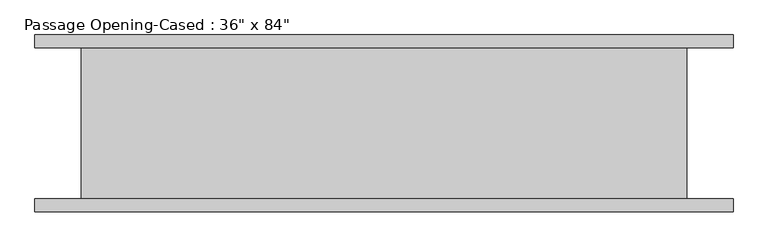
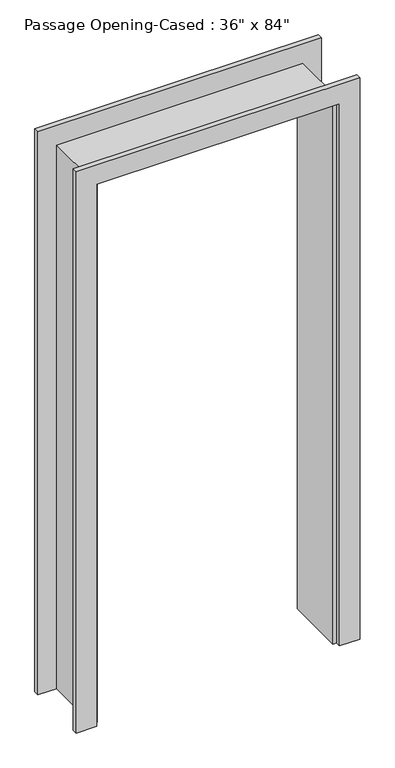
"""IFC4 building model written with IfcOpenShell, lengths in millimetres: proxy geometry."""

from ifc_helpers import new_model, si_unit, frame, origin, place, context, project, spatial, polyline, outline, extrude, faceted_brep, source, transform, mapped, element, save


def proxy_e9bf662a(model_context):
    return source(origin(), model_context, "Body", "SolidModel", [
        faceted_brep([(429.9613433, 114.3, 0.0), (449.0113433, 114.3, 0.0), (449.0113433, -114.3, 0.0), (429.9613433, -114.3, 0.0), (429.9613433, 114.3, 2114.55), (449.0113433, 114.3, 2133.6), (449.0113433, -114.3, 2133.6), (429.9613433, -114.3, 2114.55), (-446.3386567, 114.3, 2114.55), (-465.3886567, 114.3, 2133.6), (-465.3886567, -114.3, 2133.6), (-446.3386567, -114.3, 2114.55), (-446.3386567, 114.3, 0.0), (-446.3386567, -114.3, 0.0), (-465.3886567, -114.3, 0.0), (-465.3886567, 114.3, 0.0)], [[[0, 1, 2, 3]], [[1, 0, 4, 5]], [[2, 1, 5, 6]], [[3, 2, 6, 7]], [[0, 3, 7, 4]], [[5, 4, 8, 9]], [[6, 5, 9, 10]], [[7, 6, 10, 11]], [[4, 7, 11, 8]], [[12, 13, 14, 15]], [[9, 8, 12, 15]], [[10, 9, 15, 14]], [[11, 10, 14, 13]], [[8, 11, 13, 12]]]),
        extrude(outline(polyline([(0.0, 518.8613433), (2209.8, 518.8613433), (2209.8, -535.2386567), (0.0, -535.2386567), (0.0, -459.0386567), (2127.25, -459.0386567), (2127.25, 442.6613433), (0.0, 442.6613433), (0.0, 518.8613433)])), frame((0.0, 114.3, 0.0), z_axis=(0.0, 1.0, 0.0), x_axis=(0.0, 0.0, 1.0)), (0.0, 0.0, 1.0), 19.05),
        extrude(outline(polyline([(0.0, -459.0386567), (2127.25, -459.0386567), (2127.25, 442.6613433), (0.0, 442.6613433), (0.0, 518.8613433), (2203.45, 518.8613433), (2203.45, -535.2386567), (0.0, -535.2386567), (0.0, -459.0386567)])), frame((0.0, -133.35, 0.0), z_axis=(0.0, 1.0, 0.0), x_axis=(0.0, 0.0, 1.0)), (0.0, 0.0, 1.0), 19.05),
    ])


if __name__ == "__main__":
    model = new_model("IFC4")
    model_context = context("Model", 3, world=origin())
    ifc_project = project(units=[si_unit("LENGTHUNIT", "METRE", prefix="MILLI")], contexts=[model_context])
    site = spatial("IfcSite", under=ifc_project)
    building = spatial("IfcBuilding", under=site)
    placement = place(None, origin())
    proxy_shape = proxy_e9bf662a(model_context)
    element("IfcBuildingElementProxy", 1, Name="Passage Opening-Cased : 36\" x 84\"", ObjectType="Passage Opening-Cased : 36\" x 84\"", at=placement, inside=building, context=model_context, shape_type="MappedRepresentation", body=[
        mapped(proxy_shape, transform((0.0, 0.0, 0.0), x_axis=(1.0, 0.0, 0.0), y_axis=(0.0, 1.0, 0.0), z_axis=(0.0, 0.0, 1.0))),
    ])
    save(model, "model.ifc")

# Revit data of these elements
# Type "Passage Opening-Cased : 36\" x 84\""
#   Height = 7' - 0"
#   Trim Thickness = 0' - 0 3/4"
#   Trim Width = 0' - 3"
#   Width = 3' - 0"
#   Frame Material = Door - Frame
#   Default Elevation = 0
# Element 1 (IfcBuildingElementProxy, "Passage Opening-Cased : 36\" x 84\"")
#   Materials on its faces: "Door - Frame"
# Materials
#   "Door - Frame": colour RGB 118 70 51, transparency 0, Cost = 0
